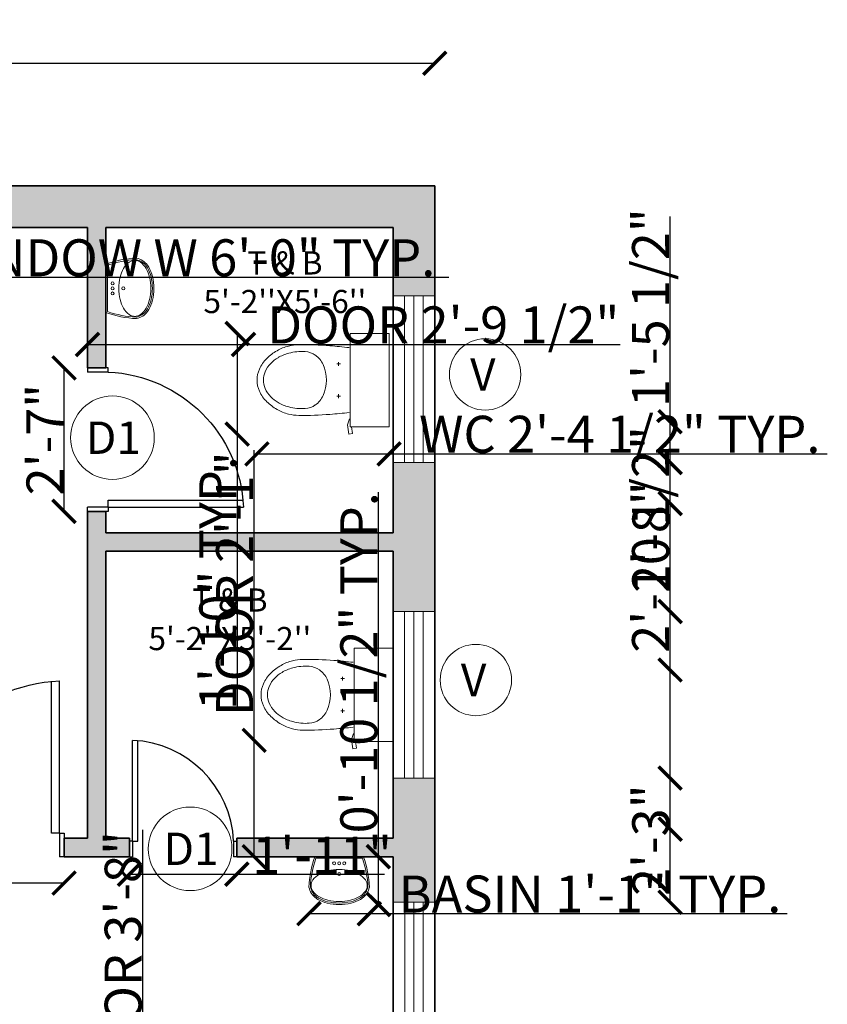
# Model space of a CAD drawing. Units: inches. Extents: x 2209 to 2954, y 1760 to 2265.
# Tile 7 of 7: x 2780 to 2954, y 2005 to 2218. Entities that reach past the tile are written whole.
import ezdxf

# ---------------------------------------------------------------- set-up
doc = ezdxf.new("R2010")
doc.units = ezdxf.units.IN
for name, color, linetype, lineweight in [('A-ANNO-DIMS', 2, 'Continuous', 18), ('A-ANNO-SYMB', 7, 'Continuous', 18), ('A-AREA-IDEN', 7, 'Continuous', 18), ('A-FLOR-FIXT', 9, 'Continuous', 18), ('A-WALL-PATT', 30, 'Continuous', 13), ('DOOR', 240, 'Continuous', 25), ('WALL', 7, 'Continuous', 35), ('WINDOW', 190, 'Continuous', 18)]:
    doc.layers.add(name, color=color, linetype=linetype, lineweight=lineweight)
doc.styles.get("Standard").update_dxf_attribs({"font": 'arial.ttf'})
doc.dimstyles.get("Standard").update_dxf_attribs({"dimtxt": 8, "dimasz": 5, "dimexe": 0.18, "dimexo": 0.0625, "dimgap": 0.09, "dimtad": 1, "dimdec": 1, "dimzin": 0, "dimdsep": 46, "dimlunit": 4, "dimtxsty": 'Standard', "dimblk": 'ARCHTICK', "dimcen": 0.09, "dimse1": 1, "dimse2": 1, "dimadec": 0, "dimazin": 0, "dimtfac": 1, "dimtdec": 1, "dimtofl": 0, "dimtmove": 0, "dimatfit": 3, "dimfxl": 1, "dimtolj": 1, "dimtzin": 0, "dimarcsym": 0})

# ---------------------------------------------------------------- blocks, each defined once
blk = doc.blocks.new('AP0B05')
for p, q in [((35, 100), (35, 880)), ((75, 100), (75, 878.9)), ((35, 100), (11, 100)), ((11, 100), (11, -20)), ((35, 100), (35, -20)), ((815, 100), (815, -20)), ((815, 100), (839, 100)), ((839, 100), (839, -20)), ((11, -20), (35, -20)), ((839, -20), (815, -20))]:
    blk.add_line(p, q)
blk.add_lwpolyline([(35, 100), (75, 100)])
blk.add_arc((-2.4, 62.6), 818.3, 2.6212, 87.3788)
blk = doc.blocks.new('toilet-1')
at = {"color": 0, "linetype": 'ByBlock'}
for p, q in [((-0.23, -0.02), (-0.23, -0.2116)), ((0.23, -0.02), (-0.23, -0.02)), ((0.23, -0.02), (0.23, -0.2116)), ((-0.23, -0.2116), (0.23, -0.2116)), ((0.1917, -0.2144), (0.2206, -0.225)), ((0.2206, -0.225), (0.266, -0.2187)), ((0.2633, -0.1997), (0.23, -0.2044)), ((0.266, -0.2187), (0.2633, -0.1997)), ((-0.0889, -0.2683), (-0.0697, -0.2683)), ((-0.0793, -0.2587), (-0.0793, -0.2778)), ((0.0889, -0.2683), (0.0698, -0.2683)), ((0.0794, -0.2587), (0.0794, -0.2778)), ((0, -0.6382), (0, -0.6382))]:
    blk.add_line(p, q, dxfattribs=at)
for centre, radius, start, end in [((3.5272, -0.6239), 3.7093, 173.6925, 175.1593), ((-3.527, -0.624), 3.7093, 4.8413, 6.3171), ((1.7368, -0.4519), 1.9109, 175.7698, 180.3758), ((0, -0.5169), 0.1884, 66.0939, 113.9061), ((-1.7366, -0.4519), 1.9109, 359.6242, 4.2302), ((-0.0408, -0.4398), 0.0996, 145.1497, 175.881), ((-0.0312, -0.4465), 0.1114, 113.8997, 145.1485), ((0.0312, -0.4465), 0.1114, 34.8515, 66.1003), ((0.0409, -0.4398), 0.0996, 4.119, 34.8503), ((0.0981, -0.4497), 0.2389, 175.8862, 195.5931), ((-0.098, -0.4497), 0.2389, 344.4069, 4.1138), ((0.0353, -0.463), 0.2093, 180.3747, 194.3375), ((-0.0351, -0.463), 0.2093, 345.6614, 359.6243), ((0.055, -0.458), 0.2297, 194.3353, 209.622), ((0.0961, -0.4503), 0.2369, 195.5969, 209.3771), ((-0.096, -0.4503), 0.2369, 330.6229, 344.4031), ((-0.0548, -0.458), 0.2297, 330.3788, 345.6655), ((0.0647, -0.4524), 0.2409, 209.6273, 224.5489), ((0.0232, -0.4913), 0.1532, 209.3871, 226.5438), ((-0.0231, -0.4913), 0.1532, 313.4562, 330.6129), ((-0.0645, -0.4524), 0.2409, 315.4504, 330.372), ((0.0178, -0.4986), 0.1751, 224.552, 245.714), ((0.0152, -0.4997), 0.1416, 226.5501, 246.5527), ((0, -0.5347), 0.1034, 246.5493, 270.0042), ((0, -0.5347), 0.1034, 269.9958, 293.4507), ((-0.0151, -0.4997), 0.1416, 293.4473, 313.4499), ((-0.0176, -0.4986), 0.1751, 294.2865, 315.4485), ((0.0004, -0.538), 0.132, 245.5845, 269.8782), ((-0.0002, -0.538), 0.132, 270.1216, 294.4153)]:
    blk.add_arc(centre, radius, start, end, dxfattribs=at)
blk = doc.blocks.new('wash-3')
at = {"color": 0, "linetype": 'ByBlock'}
blk.add_line((0.2303, -0.0146), (-0.2303, -0.0146), dxfattribs=at)
for centre in [(-0.05, -0.0656), (0, -0.0656), (0.05, -0.0656), (0, -0.1721)]:
    blk.add_circle(centre, 0.0148, dxfattribs=at)
for centre, radius, start, end in [((0.6901, -0.3398), 0.9908, 159.94105, 177.83899), ((0.6901, -0.3398), 0.9762, 160.53992, 177.73258), ((-0.6901, -0.3398), 0.9762, 2.26742, 19.46008), ((-0.6901, -0.3398), 0.9908, 2.16101, 20.05895), ((-0.0958, -0.3493), 0.2026, 119.83217, 144.15878), ((-0.038, -0.4501), 0.3188, 103.36192, 119.83217), ((0, -0.6101), 0.4833, 90, 103.36192), ((0, -0.6101), 0.4833, 76.63808, 90), ((0.038, -0.4501), 0.3188, 60.16783, 76.63808), ((0.0958, -0.3493), 0.2026, 35.84122, 60.16783), ((-0.1831, -0.2863), 0.095, 144.15878, 180), ((-0.1831, -0.2863), 0.095, 180, 215.84122), ((0.1831, -0.2863), 0.095, 0, 35.84122), ((0.1831, -0.2863), 0.095, 324.15878, 0), ((-0.12, -0.2651), 0.1838, 191.74238, 233.41914), ((-0.12, -0.2651), 0.1692, 192.33583, 233.36097), ((-0.0958, -0.2233), 0.2026, 215.84122, 240.16783), ((0.0958, -0.2233), 0.2026, 299.83217, 324.15878), ((0.12, -0.2651), 0.1692, 306.63903, 347.66417), ((0.12, -0.2651), 0.1838, 306.58086, 348.25762), ((-0.0958, -0.2233), 0.2319, 234.77185, 240.16783), ((-0.0958, -0.2233), 0.2173, 234.81756, 240.16783), ((-0.038, -0.1224), 0.3481, 240.16783, 256.63808), ((-0.038, -0.1224), 0.3335, 240.16783, 256.63808), ((-0.038, -0.1224), 0.3188, 240.16783, 256.63808), ((0, 0.0376), 0.5126, 256.63808, 270), ((0, 0.0376), 0.4979, 256.63808, 270), ((0, 0.0376), 0.4833, 256.63808, 270), ((0, 0.0376), 0.4833, 270, 283.36192), ((0, 0.0376), 0.4979, 270, 283.36192), ((0, 0.0376), 0.5126, 270, 283.36192), ((0.038, -0.1224), 0.3188, 283.36192, 299.83217), ((0.038, -0.1224), 0.3335, 283.36192, 299.83217), ((0.038, -0.1224), 0.3481, 283.36192, 299.83217), ((0.0958, -0.2233), 0.2173, 299.83217, 305.18244), ((0.0958, -0.2233), 0.2319, 299.83217, 305.22815)]:
    blk.add_arc(centre, radius, start, end, dxfattribs=at)
blk = doc.blocks.new('_ArchTick')
at = {"color": 0, "linetype": 'ByBlock', "const_width": 0.15}
blk.add_lwpolyline([(-0.5, -0.5), (0.5, 0.5)], dxfattribs=at)
blk = doc.blocks.new('*D15')
at = {"layer": 'A-ANNO-DIMS', "color": 0, "lineweight": -2, "transparency": 16777216}
blk.add_line((2629.22, 2208.74), (2869.22, 2208.74), dxfattribs=at)
at = {"layer": 'Defpoints', "color": 0, "transparency": 16777216}
for p in [(2869.22, 2208.74), (2629.22, 2182.29), (2869.22, 2182.29)]:
    blk.add_point(p, dxfattribs=at)
at = {"layer": 'A-ANNO-DIMS', "color": 0, "lineweight": -2, "transparency": 16777216, "xscale": 5, "yscale": 5, "zscale": 5, "rotation": 180}
blk.add_blockref('_ArchTick', (2629.22, 2208.74), dxfattribs=at)
at = {"layer": 'A-ANNO-DIMS', "color": 0, "lineweight": -2, "transparency": 16777216, "xscale": 5, "yscale": 5, "zscale": 5}
blk.add_blockref('_ArchTick', (2869.22, 2208.74), dxfattribs=at)
at = {"layer": 'A-ANNO-DIMS', "color": 0, "transparency": 16777216, "insert": (2749.22, 2212.91), "char_height": 8, "attachment_point": 5}
blk.add_mtext("\\A1;20'", dxfattribs=at)
blk = doc.blocks.new('WIN-W-72IN')
for p, q in [((0, 6.5), (72, 6.5)), ((0, 4.5), (72, 4.5)), ((0, 2.5), (72, 2.5))]:
    blk.add_line(p, q)
blk.add_lwpolyline([(0, 9), (72, 9), (72, 0), (0, 0)], close=True)
blk = doc.blocks.new('VENT-V-36IN')
for p, q in [((2.5, 0), (2.5, 36)), ((4.5, 0), (4.5, 36)), ((6.5, 0), (6.5, 36))]:
    blk.add_line(p, q)
blk.add_lwpolyline([(0, 0), (0, 36), (9, 36), (9, 0)], close=True)
blk = doc.blocks.new('TAG-OPENING-V')
blk.add_circle((0, 0), 7.71)
blk.add_text('V', height=7).set_placement((-3.24, -3.5))
blk = doc.blocks.new('TAG-OPENING-D1')
blk.add_circle((0, 0), 9.03)
blk.add_text('D1', height=7).set_placement((-5.73, -3.51))
blk = doc.blocks.new('*D27')
at = {"layer": 'A-ANNO-DIMS', "color": 0, "lineweight": -2, "transparency": 16777216}
for p, q in [((2680.22, 2162.49), (2752.22, 2162.49)), ((2752.22, 2162.49), (2872.28, 2162.49))]:
    blk.add_line(p, q, dxfattribs=at)
at = {"layer": 'Defpoints', "color": 0, "transparency": 16777216}
for p in [(2680.22, 2173.29), (2752.22, 2173.29), (2752.22, 2162.49)]:
    blk.add_point(p, dxfattribs=at)
at = {"layer": 'A-ANNO-DIMS', "color": 0, "lineweight": -2, "transparency": 16777216, "xscale": 5, "yscale": 5, "zscale": 5, "rotation": 180}
blk.add_blockref('_ArchTick', (2680.22, 2162.49), dxfattribs=at)
at = {"layer": 'A-ANNO-DIMS', "color": 0, "lineweight": -2, "transparency": 16777216, "xscale": 5, "yscale": 5, "zscale": 5}
blk.add_blockref('_ArchTick', (2752.22, 2162.49), dxfattribs=at)
at = {"layer": 'A-ANNO-DIMS', "color": 0, "transparency": 16777216, "insert": (2814.75, 2166.71), "char_height": 8, "attachment_point": 5}
blk.add_mtext('\\A1;WINDOW W 6\'-0" TYP.', dxfattribs=at)
blk = doc.blocks.new('*D33')
at = {"layer": 'A-ANNO-DIMS', "color": 0, "lineweight": -2, "transparency": 16777216}
for p, q in [((2830.22, 2062.44), (2830.22, 2125.12)), ((2830.22, 2037.29), (2830.22, 2062.44))]:
    blk.add_line(p, q, dxfattribs=at)
at = {"layer": 'Defpoints', "color": 0, "transparency": 16777216}
for p in [(2826.45, 2062.44), (2830.22, 2062.44), (2826.45, 2037.29)]:
    blk.add_point(p, dxfattribs=at)
at = {"layer": 'A-ANNO-DIMS', "color": 0, "lineweight": -2, "transparency": 16777216, "xscale": 5, "yscale": 5, "zscale": 5}
for p, rotation in [((2830.22, 2062.44), 90), ((2830.22, 2037.29), 270)]:
    blk.add_blockref('_ArchTick', p, dxfattribs=dict(at, rotation=rotation))
at = {"layer": 'A-ANNO-DIMS', "color": 0, "transparency": 16777216, "insert": (2825.99, 2096.28), "char_height": 8, "attachment_point": 5, "rotation": 90}
blk.add_mtext('\\A1;DOOR 2\'-1"', dxfattribs=at)
blk = doc.blocks.new('*D34')
at = {"layer": 'A-ANNO-DIMS', "color": 0, "lineweight": -2, "transparency": 16777216}
for p, q in [((2803.31, 2033.51), (2826.45, 2033.51)), ((2826.45, 2033.51), (2858.36, 2033.51))]:
    blk.add_line(p, q, dxfattribs=at)
at = {"layer": 'Defpoints', "color": 0, "transparency": 16777216}
for p in [(2803.31, 2037.29), (2826.45, 2037.29), (2826.45, 2033.51)]:
    blk.add_point(p, dxfattribs=at)
at = {"layer": 'A-ANNO-DIMS', "color": 0, "lineweight": -2, "transparency": 16777216, "xscale": 5, "yscale": 5, "zscale": 5, "rotation": 180}
blk.add_blockref('_ArchTick', (2803.31, 2033.51), dxfattribs=at)
at = {"layer": 'A-ANNO-DIMS', "color": 0, "lineweight": -2, "transparency": 16777216, "xscale": 5, "yscale": 5, "zscale": 5}
blk.add_blockref('_ArchTick', (2826.45, 2033.51), dxfattribs=at)
at = {"layer": 'A-ANNO-DIMS', "color": 0, "transparency": 16777216, "insert": (2844.9, 2037.62), "char_height": 8, "attachment_point": 5}
blk.add_mtext('\\A1;1\'-11"', dxfattribs=at)
blk = doc.blocks.new('*D38')
at = {"layer": 'A-ANNO-DIMS', "color": 0, "lineweight": -2, "transparency": 16777216}
for p, q in [((2754.22, 2031.59), (2693.92, 2031.59)), ((2789.17, 2031.59), (2754.22, 2031.59))]:
    blk.add_line(p, q, dxfattribs=at)
at = {"layer": 'Defpoints', "color": 0, "transparency": 16777216}
for p in [(2754.22, 2037.29), (2789.17, 2037.29), (2754.22, 2031.59)]:
    blk.add_point(p, dxfattribs=at)
at = {"layer": 'A-ANNO-DIMS', "color": 0, "lineweight": -2, "transparency": 16777216, "xscale": 5, "yscale": 5, "zscale": 5, "rotation": 180}
blk.add_blockref('_ArchTick', (2754.22, 2031.59), dxfattribs=at)
at = {"layer": 'A-ANNO-DIMS', "color": 0, "lineweight": -2, "transparency": 16777216, "xscale": 5, "yscale": 5, "zscale": 5}
blk.add_blockref('_ArchTick', (2789.17, 2031.59), dxfattribs=at)
at = {"layer": 'A-ANNO-DIMS', "color": 0, "transparency": 16777216, "insert": (2721.57, 2035.7), "char_height": 8, "attachment_point": 5}
blk.add_mtext('\\A1;2\'-11" TYP.', dxfattribs=at)
blk = doc.blocks.new('*D39')
at = {"layer": 'A-ANNO-DIMS', "color": 0, "lineweight": -2, "transparency": 16777216}
for p, q in [((2806.16, 1980.39), (2806.16, 2043.07)), ((2806.16, 1936.29), (2806.16, 1980.39))]:
    blk.add_line(p, q, dxfattribs=at)
at = {"layer": 'Defpoints', "color": 0, "transparency": 16777216}
for p in [(2806.16, 1980.39), (2812.78, 1980.39), (2812.78, 1936.29)]:
    blk.add_point(p, dxfattribs=at)
at = {"layer": 'A-ANNO-DIMS', "color": 0, "lineweight": -2, "transparency": 16777216, "xscale": 5, "yscale": 5, "zscale": 5}
for p, rotation in [((2806.16, 1980.39), 90), ((2806.16, 1936.29), 270)]:
    blk.add_blockref('_ArchTick', p, dxfattribs=dict(at, rotation=rotation))
at = {"layer": 'A-ANNO-DIMS', "color": 0, "transparency": 16777216, "insert": (2801.93, 2014.23), "char_height": 8, "attachment_point": 5, "rotation": 90}
blk.add_mtext('\\A1;DOOR 3\'-8"', dxfattribs=at)
blk = doc.blocks.new('*D41')
at = {"layer": 'A-ANNO-DIMS', "color": 0, "lineweight": -2, "transparency": 16777216}
for p, q in [((2794.22, 2147.97), (2827.91, 2147.97)), ((2827.91, 2147.97), (2909.23, 2147.97))]:
    blk.add_line(p, q, dxfattribs=at)
at = {"layer": 'Defpoints', "color": 0, "transparency": 16777216}
for p in [(2827.91, 2147.97), (2794.22, 2142.92), (2827.91, 2142.92)]:
    blk.add_point(p, dxfattribs=at)
at = {"layer": 'A-ANNO-DIMS', "color": 0, "lineweight": -2, "transparency": 16777216, "xscale": 5, "yscale": 5, "zscale": 5, "rotation": 180}
blk.add_blockref('_ArchTick', (2794.22, 2147.97), dxfattribs=at)
at = {"layer": 'A-ANNO-DIMS', "color": 0, "lineweight": -2, "transparency": 16777216, "xscale": 5, "yscale": 5, "zscale": 5}
blk.add_blockref('_ArchTick', (2827.91, 2147.97), dxfattribs=at)
at = {"layer": 'A-ANNO-DIMS', "color": 0, "transparency": 16777216, "insert": (2871.07, 2152.2), "char_height": 8, "attachment_point": 5}
blk.add_mtext('\\A1;DOOR 2\'-9 1/2"', dxfattribs=at)
blk = doc.blocks.new('*D42')
at = {"layer": 'A-ANNO-DIMS', "color": 0, "lineweight": -2, "transparency": 16777216}
blk.add_line((2789.16, 2111.92), (2789.16, 2142.92), dxfattribs=at)
at = {"layer": 'Defpoints', "color": 0, "transparency": 16777216}
for p in [(2789.16, 2142.92), (2794.22, 2142.92), (2794.22, 2111.92)]:
    blk.add_point(p, dxfattribs=at)
at = {"layer": 'A-ANNO-DIMS', "color": 0, "lineweight": -2, "transparency": 16777216, "xscale": 5, "yscale": 5, "zscale": 5}
for p, rotation in [((2789.16, 2142.92), 90), ((2789.16, 2111.92), 270)]:
    blk.add_blockref('_ArchTick', p, dxfattribs=dict(at, rotation=rotation))
at = {"layer": 'A-ANNO-DIMS', "color": 0, "transparency": 16777216, "insert": (2785.05, 2127.42), "char_height": 8, "attachment_point": 5, "rotation": 90}
blk.add_mtext('\\A1;2\'-7"', dxfattribs=at)
blk = doc.blocks.new('*D55')
at = {"layer": 'A-ANNO-DIMS', "color": 0, "lineweight": -2, "transparency": 16777216}
for p, q in [((2830.82, 2124.34), (2859.34, 2124.34)), ((2859.34, 2124.34), (2953.97, 2124.34))]:
    blk.add_line(p, q, dxfattribs=at)
at = {"layer": 'Defpoints', "color": 0, "transparency": 16777216}
for p in [(2830.82, 2128.62), (2859.34, 2128.62), (2859.34, 2124.34)]:
    blk.add_point(p, dxfattribs=at)
at = {"layer": 'A-ANNO-DIMS', "color": 0, "lineweight": -2, "transparency": 16777216, "xscale": 5, "yscale": 5, "zscale": 5, "rotation": 180}
blk.add_blockref('_ArchTick', (2830.82, 2124.34), dxfattribs=at)
at = {"layer": 'A-ANNO-DIMS', "color": 0, "lineweight": -2, "transparency": 16777216, "xscale": 5, "yscale": 5, "zscale": 5}
blk.add_blockref('_ArchTick', (2859.34, 2124.34), dxfattribs=at)
at = {"layer": 'A-ANNO-DIMS', "color": 0, "transparency": 16777216, "insert": (2909.16, 2128.57), "char_height": 8, "attachment_point": 5}
blk.add_mtext('\\A1;WC 2\'-4 1/2" TYP.', dxfattribs=at)
blk = doc.blocks.new('*D56')
at = {"layer": 'A-ANNO-DIMS', "color": 0, "lineweight": -2, "transparency": 16777216}
for p, q in [((2826.55, 2150.37), (2826.55, 2128.62)), ((2826.55, 2128.62), (2826.55, 2069.21))]:
    blk.add_line(p, q, dxfattribs=at)
at = {"layer": 'Defpoints', "color": 0, "transparency": 16777216}
for p in [(2830.82, 2150.37), (2826.55, 2128.62), (2830.82, 2128.62)]:
    blk.add_point(p, dxfattribs=at)
at = {"layer": 'A-ANNO-DIMS', "color": 0, "lineweight": -2, "transparency": 16777216, "xscale": 5, "yscale": 5, "zscale": 5}
for p, rotation in [((2826.55, 2150.37), 90), ((2826.55, 2128.62), 270)]:
    blk.add_blockref('_ArchTick', p, dxfattribs=dict(at, rotation=rotation))
at = {"layer": 'A-ANNO-DIMS', "color": 0, "transparency": 16777216, "insert": (2822.37, 2096.41), "char_height": 8, "attachment_point": 5, "rotation": 90}
blk.add_mtext('\\A1;1\'-10" TYP.', dxfattribs=at)
blk = doc.blocks.new('*D57')
at = {"layer": 'A-ANNO-DIMS', "color": 0, "lineweight": -2, "transparency": 16777216}
for p, q in [((2842.04, 2024.99), (2855.09, 2024.99)), ((2855.09, 2024.99), (2945.32, 2024.99))]:
    blk.add_line(p, q, dxfattribs=at)
at = {"layer": 'Defpoints', "color": 0, "transparency": 16777216}
for p in [(2842.04, 2026.95), (2855.09, 2026.95), (2855.09, 2024.99)]:
    blk.add_point(p, dxfattribs=at)
at = {"layer": 'A-ANNO-DIMS', "color": 0, "lineweight": -2, "transparency": 16777216, "xscale": 5, "yscale": 5, "zscale": 5, "rotation": 180}
blk.add_blockref('_ArchTick', (2842.04, 2024.99), dxfattribs=at)
at = {"layer": 'A-ANNO-DIMS', "color": 0, "lineweight": -2, "transparency": 16777216, "xscale": 5, "yscale": 5, "zscale": 5}
blk.add_blockref('_ArchTick', (2855.09, 2024.99), dxfattribs=at)
at = {"layer": 'A-ANNO-DIMS', "color": 0, "transparency": 16777216, "insert": (2902.71, 2029.22), "char_height": 8, "attachment_point": 5}
blk.add_mtext('\\A1;BASIN 1\'-1" TYP.', dxfattribs=at)
blk = doc.blocks.new('*D58')
at = {"layer": 'A-ANNO-DIMS', "color": 0, "lineweight": -2, "transparency": 16777216}
for p, q in [((2857.05, 2037.29), (2857.05, 2116.09)), ((2857.05, 2026.95), (2857.05, 2037.29))]:
    blk.add_line(p, q, dxfattribs=at)
at = {"layer": 'Defpoints', "color": 0, "transparency": 16777216}
for p in [(2855.09, 2037.29), (2857.05, 2037.29), (2855.09, 2026.95)]:
    blk.add_point(p, dxfattribs=at)
at = {"layer": 'A-ANNO-DIMS', "color": 0, "lineweight": -2, "transparency": 16777216, "xscale": 5, "yscale": 5, "zscale": 5}
for p, rotation in [((2857.05, 2037.29), 90), ((2857.05, 2026.95), 270)]:
    blk.add_blockref('_ArchTick', p, dxfattribs=dict(at, rotation=rotation))
at = {"layer": 'A-ANNO-DIMS', "color": 0, "transparency": 16777216, "insert": (2852.82, 2079.19), "char_height": 8, "attachment_point": 5, "rotation": 90}
blk.add_mtext('\\A1;0\'-10 1/2" TYP.', dxfattribs=at)
blk = doc.blocks.new('*D76')
at = {"layer": 'A-ANNO-DIMS', "color": 0, "lineweight": -2, "transparency": 16777216}
for p, q in [((2920.04, 2077.63), (2920.04, 2129.07)), ((2920.04, 2043.25), (2920.04, 2077.63))]:
    blk.add_line(p, q, dxfattribs=at)
at = {"layer": 'Defpoints', "color": 0, "transparency": 16777216}
for p in [(2519.15, 2077.63), (2920.04, 2077.63), (2519.15, 2043.25)]:
    blk.add_point(p, dxfattribs=at)
at = {"layer": 'A-ANNO-DIMS', "color": 0, "lineweight": -2, "transparency": 16777216, "xscale": 5, "yscale": 5, "zscale": 5}
for p, rotation in [((2920.04, 2077.63), 90), ((2920.04, 2043.25), 270)]:
    blk.add_blockref('_ArchTick', p, dxfattribs=dict(at, rotation=rotation))
at = {"layer": 'A-ANNO-DIMS', "color": 0, "transparency": 16777216, "insert": (2915.82, 2105.85), "char_height": 8, "attachment_point": 5, "rotation": 90}
blk.add_mtext('\\A1;2\'-10 1/2"', dxfattribs=at)
blk = doc.blocks.new('*D77')
at = {"layer": 'A-ANNO-DIMS', "color": 0, "lineweight": -2, "transparency": 16777216}
for p, q in [((2920.04, 2131.29), (2920.04, 2175.62)), ((2920.04, 2113.63), (2920.04, 2131.29))]:
    blk.add_line(p, q, dxfattribs=at)
at = {"layer": 'Defpoints', "color": 0, "transparency": 16777216}
for p in [(2519.15, 2131.29), (2920.04, 2131.29), (2519.15, 2113.63)]:
    blk.add_point(p, dxfattribs=at)
at = {"layer": 'A-ANNO-DIMS', "color": 0, "lineweight": -2, "transparency": 16777216, "xscale": 5, "yscale": 5, "zscale": 5}
for p, rotation in [((2920.04, 2131.29), 90), ((2920.04, 2113.63), 270)]:
    blk.add_blockref('_ArchTick', p, dxfattribs=dict(at, rotation=rotation))
at = {"layer": 'A-ANNO-DIMS', "color": 0, "transparency": 16777216, "insert": (2915.82, 2155.95), "char_height": 8, "attachment_point": 5, "rotation": 90}
blk.add_mtext('\\A1;1\'-5 1/2"', dxfattribs=at)
blk = doc.blocks.new('*D91')
at = {"layer": 'A-ANNO-DIMS', "color": 0, "lineweight": -2, "transparency": 16777216}
blk.add_line((2920.04, 2027.43), (2920.04, 2054.29), dxfattribs=at)
at = {"layer": 'Defpoints', "color": 0, "transparency": 16777216}
for p in [(2869.22, 2054.29), (2920.04, 2054.29), (2869.22, 2027.43)]:
    blk.add_point(p, dxfattribs=at)
at = {"layer": 'A-ANNO-DIMS', "color": 0, "lineweight": -2, "transparency": 16777216, "xscale": 5, "yscale": 5, "zscale": 5}
for p, rotation in [((2920.04, 2054.29), 90), ((2920.04, 2027.43), 270)]:
    blk.add_blockref('_ArchTick', p, dxfattribs=dict(at, rotation=rotation))
at = {"layer": 'A-ANNO-DIMS', "color": 0, "transparency": 16777216, "insert": (2915.86, 2040.86), "char_height": 8, "attachment_point": 5, "rotation": 90}
blk.add_mtext('\\A1;2\'-3"', dxfattribs=at)
blk = doc.blocks.new('*D92')
at = {"layer": 'A-ANNO-DIMS', "color": 0, "lineweight": -2, "transparency": 16777216}
blk.add_line((2920.04, 2090.29), (2920.04, 2122.46), dxfattribs=at)
at = {"layer": 'Defpoints', "color": 0, "transparency": 16777216}
for p in [(2869.22, 2122.46), (2920.04, 2122.46), (2869.22, 2090.29)]:
    blk.add_point(p, dxfattribs=at)
at = {"layer": 'A-ANNO-DIMS', "color": 0, "lineweight": -2, "transparency": 16777216, "xscale": 5, "yscale": 5, "zscale": 5}
for p, rotation in [((2920.04, 2122.46), 90), ((2920.04, 2090.29), 270)]:
    blk.add_blockref('_ArchTick', p, dxfattribs=dict(at, rotation=rotation))
at = {"layer": 'A-ANNO-DIMS', "color": 0, "transparency": 16777216, "insert": (2915.87, 2106.37), "char_height": 8, "attachment_point": 5, "rotation": 90}
blk.add_mtext('\\A1;2\'-8"', dxfattribs=at)
blk = doc.blocks.new('*D93')
at = {"layer": 'A-ANNO-DIMS', "color": 0, "lineweight": -2, "transparency": 16777216}
for p, q in [((2224.78, 2107.29), (2224.78, 2133.73)), ((2224.78, 2103.29), (2224.78, 2107.29))]:
    blk.add_line(p, q, dxfattribs=at)
at = {"layer": 'Defpoints', "color": 0, "transparency": 16777216}
for p in [(2224.78, 2107.29), (2798.22, 2107.29), (2798.22, 2103.29)]:
    blk.add_point(p, dxfattribs=at)
at = {"layer": 'A-ANNO-DIMS', "color": 0, "lineweight": -2, "transparency": 16777216, "xscale": 5, "yscale": 5, "zscale": 5}
for p, rotation in [((2224.78, 2107.29), 90), ((2224.78, 2103.29), 270)]:
    blk.add_blockref('_ArchTick', p, dxfattribs=dict(at, rotation=rotation))
at = {"layer": 'A-ANNO-DIMS', "color": 0, "transparency": 16777216, "insert": (2220.61, 2123.01), "char_height": 8, "attachment_point": 5, "rotation": 90}
blk.add_mtext('\\A1;0\'-4"', dxfattribs=at)

msp = doc.modelspace()

# ---------------------------------------------------------------- hatches: boundary and pattern name
at = {"layer": 'A-WALL-PATT', "transparency": 33554585}
h = msp.add_hatch(color=256, dxfattribs=at)
h.dxf.hatch_style = 1
h.paths.add_polyline_path([(2519.15, 2182.29), (2402.15, 2182.29), (2402.15, 2173.29), (2444.15, 2173.29), (2444.15, 2154.12), (2448.15, 2154.12), (2448.15, 2173.29), (2510.15, 2173.29), (2510.15, 2167.29), (2519.15, 2167.29)])
h.paths.add_polyline_path([(2330.15, 2182.29), (2279.15, 2182.29), (2279.15, 2145.83), (2288.15, 2145.83), (2288.15, 2158.01), (2288.15, 2173.29), (2330.15, 2173.29)])
h.paths.add_polyline_path([(2288.15, 2073.83), (2279.15, 2073.83), (2279.15, 2009.29), (2288.15, 2009.29), (2288.15, 2037.29), (2404.15, 2037.29), (2404.15, 2041.29), (2288.15, 2041.29)])
h.paths.add_polyline_path([(2519.15, 2131.29), (2510.15, 2131.29), (2510.15, 2125.29), (2444.15, 2125.29), (2444.15, 2041.29), (2439.11, 2041.29), (2439.11, 2037.29), (2448.15, 2037.29), (2448.15, 2069.29), (2481.65, 2069.29), (2481.65, 2073.29), (2448.15, 2073.29), (2448.15, 2121.29), (2468.19, 2121.29), (2468.19, 2121.32), (2488.37, 2121.32), (2510.15, 2121.29), (2510.15, 2113.63), (2519.15, 2113.63)])
h.paths.add_polyline_path([(2519.15, 2077.63), (2510.15, 2077.63), (2510.15, 2073.32), (2510.17, 2073.32), (2510.15, 2069.19), (2510.15, 2043.25), (2519.15, 2043.25)], flags=17)
h.paths.add_polyline_path([(2519.15, 1971.25), (2510.15, 1971.25), (2510.15, 1945.29), (2444.15, 1945.29), (2444.15, 1937.21), (2448.15, 1937.21), (2448.15, 1941.29), (2510.15, 1941.29), (2510.15, 1922.29), (2519.15, 1922.29)])
h.paths.add_polyline_path([(2288.15, 1941.29), (2394.15, 1941.29), (2394.15, 1945.29), (2288.15, 1945.29), (2288.15, 1973.29), (2279.15, 1973.29), (2279.15, 1919.97), (2288.15, 1919.97)])
h.paths.add_polyline_path([(2300.65, 1831.29), (2288.15, 1831.29), (2288.15, 1847.97), (2279.15, 1847.97), (2279.15, 1822.29), (2300.65, 1822.29)])
h.paths.add_polyline_path([(2394.15, 1825.29), (2394.15, 1831.29), (2372.65, 1831.29), (2372.65, 1822.29), (2394.15, 1822.29)])
h.paths.add_polyline_path([(2449.17, 1831.29), (2448.15, 1831.29), (2448.15, 1899.32), (2444.15, 1899.32), (2444.15, 1831.29), (2439.18, 1831.29), (2439.18, 1822.29), (2449.17, 1822.29)])
h.paths.add_polyline_path([(2519.15, 1850.29), (2510.15, 1850.29), (2510.15, 1831.29), (2509.17, 1831.29), (2509.17, 1822.29), (2519.15, 1822.29)])
h.paths.add_polyline_path([(2638.22, 1941.29), (2744.22, 1941.29), (2744.22, 1945.29), (2638.22, 1945.29), (2638.22, 1973.14), (2629.22, 1973.14), (2629.22, 1919.53), (2638.22, 1919.53)])
h.paths.add_polyline_path([(2638.22, 1847.53), (2629.22, 1847.53), (2629.22, 1822.29), (2650.72, 1822.29), (2650.72, 1831.29), (2638.22, 1831.29)])
h.paths.add_polyline_path([(2638.22, 2037.29), (2754.22, 2037.29), (2754.22, 2041.29), (2638.22, 2041.29), (2638.22, 2074.27), (2629.22, 2074.27), (2629.22, 2009.14), (2638.22, 2009.14)])
h.paths.add_polyline_path([(2803.22, 1936.29), (2812.78, 1936.29), (2812.78, 1945.29), (2791.22, 1945.29), (2791.22, 1936.29), (2794.22, 1936.29), (2794.22, 1831.29), (2722.72, 1831.29), (2722.72, 1822.29), (2803.22, 1822.29)])
h.paths.add_polyline_path([(2869.22, 1955.43), (2860.22, 1955.43), (2860.22, 1945.29), (2853.36, 1945.29), (2853.36, 1936.29), (2869.22, 1936.29)])
h.paths.add_polyline_path([(2680.22, 2182.29), (2629.22, 2182.29), (2629.22, 2146.27), (2638.22, 2146.27), (2638.22, 2173.29), (2680.22, 2173.29)])
h.paths.add_polyline_path([(2869.22, 2182.29), (2752.22, 2182.29), (2752.22, 2173.29), (2794.22, 2173.29), (2794.22, 2142.92), (2798.22, 2142.92), (2798.22, 2173.29), (2860.22, 2173.29), (2860.22, 2158.46), (2869.22, 2158.46)])
h.paths.add_polyline_path([(2869.22, 2122.46), (2860.22, 2122.46), (2860.22, 2090.29), (2869.22, 2090.29)])
h = msp.add_hatch(color=256, dxfattribs=at)
h.dxf.hatch_style = 1
h.paths.add_polyline_path([(2860.22, 2107.29), (2798.22, 2107.29), (2798.22, 2111.92), (2794.22, 2111.92), (2794.22, 2041.29), (2789.17, 2041.29), (2789.17, 2037.29), (2798.22, 2037.29), (2803.31, 2037.29), (2803.31, 2041.29), (2798.22, 2041.29), (2798.22, 2103.29), (2860.22, 2103.29)])
h = msp.add_hatch(color=256, dxfattribs=at)
h.dxf.hatch_style = 1
h.paths.add_polyline_path([(2869.22, 2054.29), (2860.22, 2054.29), (2860.22, 2041.29), (2826.45, 2041.29), (2826.45, 2037.29), (2860.22, 2037.29), (2860.22, 2027.43), (2869.22, 2027.43)])

# ---------------------------------------------------------------- linework, layer by layer
at = {"layer": 'WALL'}
for p, q in [((2629.22, 2182.29), (2869.22, 2182.29)), ((2869.22, 2182.29), (2869.22, 1822.29)), ((2638.22, 2173.29), (2794.22, 2173.29)), ((2794.22, 2173.29), (2794.22, 2142.92)), ((2798.22, 2173.29), (2860.22, 2173.29)), ((2798.22, 2173.29), (2798.22, 2142.92)), ((2860.22, 2173.29), (2860.22, 2107.29)), ((2794.22, 2142.92), (2798.22, 2142.92)), ((2798.22, 2111.92), (2794.22, 2111.92)), ((2794.22, 2111.92), (2794.22, 2041.29)), ((2798.22, 2111.92), (2798.22, 2107.29)), ((2798.22, 2107.29), (2860.22, 2107.29)), ((2798.22, 2103.29), (2860.22, 2103.29)), ((2798.22, 2103.29), (2798.22, 2041.29)), ((2860.22, 2103.29), (2860.22, 2041.29)), ((2789.17, 2041.29), (2794.22, 2041.29)), ((2789.17, 2041.29), (2789.17, 2037.29)), ((2798.22, 2041.29), (2803.31, 2041.29)), ((2803.31, 2041.29), (2803.31, 2037.29)), ((2826.45, 2041.29), (2826.45, 2037.29)), ((2826.45, 2041.29), (2860.22, 2041.29)), ((2789.17, 2037.29), (2798.22, 2037.29)), ((2798.22, 2037.29), (2803.31, 2037.29)), ((2826.45, 2037.29), (2860.22, 2037.29)), ((2860.22, 2037.29), (2860.22, 1945.29))]:
    msp.add_line(p, q, dxfattribs=at)

# ---------------------------------------------------------------- block references
at = {"layer": 'A-ANNO-SYMB'}
for name, p in [('TAG-OPENING-V', (2880.09, 2141.51)), ('TAG-OPENING-D1', (2799.62, 2127.84)), ('TAG-OPENING-V', (2878.09, 2075.47)), ('TAG-OPENING-D1', (2816.39, 2039))]:
    msp.add_blockref(name, p, dxfattribs=at)
at = {"layer": 'A-FLOR-FIXT'}
for name, p, xscale, yscale, zscale, rotation in [('wash-3', (2798.22, 2160.1), 21.75271524526245, 21.75271524526245, 21.75271524526245, 90), ('toilet-1', (2860.22, 2140.29), 43.86874267633562, 43.86874267633562, 43.86874267633562, 270), ('toilet-1', (2861.09, 2072.29), 43.86874267633562, 43.86874267633562, 43.86874267633562, 270)]:
    msp.add_blockref(name, p, dxfattribs=dict(at, xscale=xscale, yscale=yscale, zscale=zscale, rotation=rotation))
at = {"layer": 'A-FLOR-FIXT', "xscale": 21.75271524526245, "yscale": 21.75271524526245, "zscale": 21.75271524526245}
msp.add_blockref('wash-3', (2848.57, 2037.29), dxfattribs=at)
at = {"layer": 'DOOR', "xscale": -0.037435508398338, "yscale": 0.037435508398338, "zscale": 0.037435508398338, "rotation": 270}
msp.add_blockref('AP0B05', (2794.96, 2111.51), dxfattribs=at)
at = {"layer": 'DOOR'}
for p, xscale, yscale, zscale in [((2789.63, 2038.13), -0.0422149343000152, 0.0422149343000152, 0.0422149343000152), ((2803, 2037.84), 0.027947166109813, 0.027947166109813, 0.027947166109813)]:
    msp.add_blockref('AP0B05', p, dxfattribs=dict(at, xscale=xscale, yscale=yscale, zscale=zscale))
at = {"layer": 'WINDOW'}
for p in [(2860.21, 2122.46), (2860.21, 2054.29)]:
    msp.add_blockref('VENT-V-36IN', p, dxfattribs=at)
at = {"layer": 'WINDOW', "rotation": 89.99999999999972}
msp.add_blockref('WIN-W-72IN', (2869.22, 1955.43), dxfattribs=at)

# ---------------------------------------------------------------- texts
at = {"layer": 'A-AREA-IDEN', "char_height": 5, "attachment_point": 1}
for s, insert in [("\\pxqc;T & B\\P5'-2''X5'-6''", (2814.28, 2168.1)), ("\\pxqc;T & B\\P5'-2''X5'-2''", (2802.4, 2095.26))]:
    msp.add_mtext_dynamic_manual_height_columns(s, width=45.1409, gutter_width=12.5, heights=[0], dxfattribs=dict(at, insert=insert))

# ---------------------------------------------------------------- dimensions: what is measured, and where the dimension line sits
at = {"layer": 'A-ANNO-DIMS'}
for base, p1, p2, override, picture, middle in [((2869.22, 2208.74), (2629.22, 2182.29), (2869.22, 2182.29), {"dimclrd": 0, "dimclre": 0, "dimclrt": 0}, '*D15', (2749.22, 2212.91)), ((2826.45, 2033.51), (2803.31, 2037.29), (2826.45, 2037.29), {"dimdec": 1, "dimlfac": 1, "dimrnd": 0, "dimzin": 1, "dimdsep": 46, "dimlunit": 4, "dimfrac": 2}, '*D34', (2844.9, 2037.62))]:
    dim = msp.add_linear_dim(base=base, p1=p1, p2=p2, dimstyle='Standard', override=override, dxfattribs=at)
    dim.commit()
    dim.dimension.update_dxf_attribs({"geometry": picture, "text_midpoint": middle})
for base, p1, p2, text, picture, middle in [((2752.22, 2162.49), (2680.22, 2173.29), (2752.22, 2173.29), 'WINDOW W <> TYP.', '*D27', (2814.75, 2166.71)), ((2827.91, 2147.97), (2794.22, 2142.92), (2827.91, 2142.92), 'DOOR <>', '*D41', (2871.07, 2152.2)), ((2859.34, 2124.34), (2830.82, 2128.62), (2859.34, 2128.62), 'WC <> TYP.', '*D55', (2909.16, 2128.57)), ((2855.0911, 2024.9949), (2842.0395, 2026.9526), (2855.0911, 2026.9526), 'BASIN <> TYP.', '*D57', (2902.7077, 2029.2213))]:
    dim = msp.add_linear_dim(base=base, p1=p1, p2=p2, text=text, dimstyle='Standard', override={"dimdec": 1, "dimlfac": 1, "dimrnd": 0, "dimzin": 1, "dimdsep": 46, "dimlunit": 4, "dimfrac": 2}, dxfattribs=at)
    dim.commit()
    dim.dimension.update_dxf_attribs({"geometry": picture, "text_midpoint": middle})
for base, p1, p2, picture, middle in [((2920.04, 2131.29), (2519.15, 2113.63), (2519.15, 2131.29), '*D77', (2915.82, 2155.95)), ((2789.16, 2142.92), (2794.22, 2111.92), (2794.22, 2142.92), '*D42', (2785.05, 2127.42)), ((2224.78, 2107.29), (2798.22, 2103.29), (2798.22, 2107.29), '*D93', (2220.61, 2123.01)), ((2920.04, 2077.63), (2519.15, 2043.25), (2519.15, 2077.63), '*D76', (2915.82, 2105.85)), ((2920.04, 2122.46), (2869.22, 2090.29), (2869.22, 2122.46), '*D92', (2915.87, 2106.37)), ((2920.04, 2054.29), (2869.22, 2027.43), (2869.22, 2054.29), '*D91', (2915.86, 2040.86))]:
    dim = msp.add_linear_dim(base=base, p1=p1, p2=p2, angle=90, dimstyle='Standard', override={"dimdec": 1, "dimlfac": 1, "dimrnd": 0, "dimzin": 1, "dimdsep": 46, "dimlunit": 4, "dimfrac": 2}, dxfattribs=at)
    dim.commit()
    dim.dimension.update_dxf_attribs({"geometry": picture, "text_midpoint": middle})
for base, p1, p2, angle, text, picture, middle in [((2826.5459, 2128.616), (2830.8231, 2150.375), (2830.8231, 2128.616), 270, '<> TYP.', '*D56', (2822.3713, 2096.4128)), ((2830.2209, 2062.4376), (2826.4481, 2037.2851), (2826.4481, 2062.4376), 90, 'DOOR <>', '*D33', (2825.9918, 2096.2779)), ((2857.05, 2037.29), (2855.09, 2026.95), (2855.09, 2037.29), 90, '<> TYP.', '*D58', (2852.82, 2079.19)), ((2754.2151, 2031.5861), (2789.1691, 2037.2851), (2754.2151, 2037.2851), 180, '<> TYP.', '*D38', (2721.5672, 2035.6952)), ((2806.16, 1980.39), (2812.78, 1936.29), (2812.78, 1980.39), 90, 'DOOR <>', '*D39', (2801.93, 2014.23))]:
    dim = msp.add_linear_dim(base=base, p1=p1, p2=p2, angle=angle, text=text, dimstyle='Standard', override={"dimdec": 1, "dimlfac": 1, "dimrnd": 0, "dimzin": 1, "dimdsep": 46, "dimlunit": 4, "dimfrac": 2}, dxfattribs=at)
    dim.commit()
    dim.dimension.update_dxf_attribs({"geometry": picture, "text_midpoint": middle})

doc.saveas('drawing.dxf')
